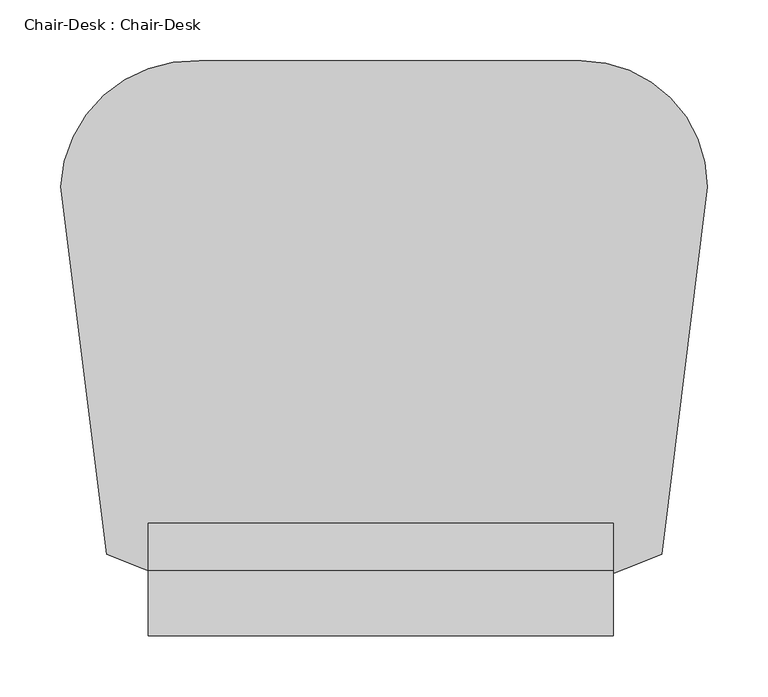
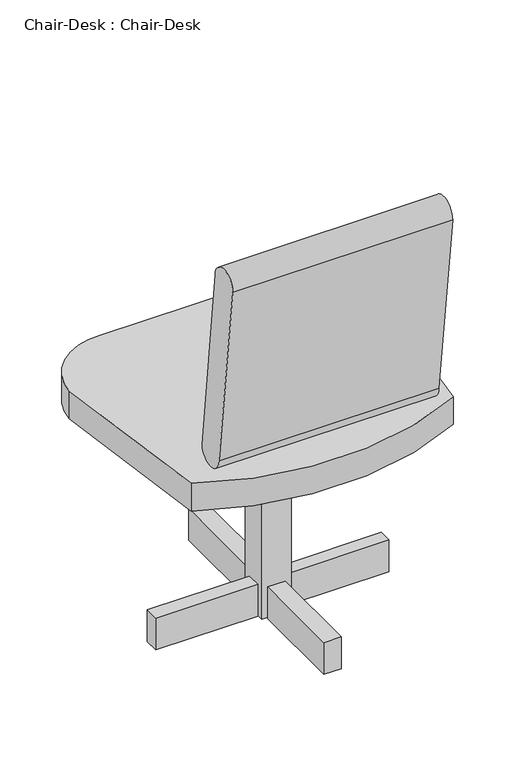
"""IFC4 building model written with IfcOpenShell, lengths in millimetres: furniture geometry, Chair-Desk : Chair-Desk."""

from ifc_helpers import new_model, si_unit, point, frame, frame_2d, origin, origin_with_axes, place, context, project, spatial, polyline, circle_curve, trimmed, segment, composite_curve, outline, extrude, source, transform, mapped, element, save


def chair_desk_chair_desk_7ad88740(model_context):
    return source(origin(), model_context, "Body", "SweptSolid", [
        extrude(outline(composite_curve([segment(trimmed(circle_curve(frame_2d((-157.1362322, 297.1024212)), 109.4001491), [point((-266.4057871, 302.4462968))], [point((-152.4, 406.4))], False, "CARTESIAN"), True, "CONTINUOUS"), segment(polyline([(-152.4, 406.4), (162.2530084, 406.4)]), True, "CONTINUOUS"), segment(trimmed(circle_curve(frame_2d((162.2530084, 302.4462968)), 103.9537032), [point((162.2530084, 406.4))], [point((266.2067116, 302.4462968))], False, "CARTESIAN"), True, "CONTINUOUS"), segment(polyline([(266.2067116, 302.4462968), (228.6, 0.0)]), True, "CONTINUOUS"), segment(trimmed(circle_curve(frame_2d((0.0, 446.8941036)), 501.9684252), [point((228.6, 0.0))], [point((-228.6, 0.0))], False, "CARTESIAN"), True, "CONTINUOUS"), segment(polyline([(-228.6, 0.0), (-266.4057871, 302.4462968)]), True, "CONTINUOUS")], self_intersect=False)), frame((0.0, 0.0, 355.6), z_axis=(0.0, 0.0, 1.0), x_axis=(1.0, 0.0, 0.0)), (0.0, 0.0, 1.0), 50.8),
        extrude(outline(composite_curve([segment(polyline([(-13.6321252, 787.4), (25.5523927, 451.3880753)]), True, "CONTINUOUS"), segment(trimmed(circle_curve(frame_2d((0.0761963, 451.3880753)), 25.4761963), [point((25.5523927, 451.3880753))], [point((-25.4, 451.3880753))], False, "CARTESIAN"), True, "CONTINUOUS"), segment(polyline([(-25.4, 451.3880753), (-67.209111, 787.4)]), True, "CONTINUOUS"), segment(trimmed(circle_curve(frame_2d((-40.4206181, 787.4)), 26.7884929), [point((-67.209111, 787.4))], [point((-13.6321252, 787.4))], False, "CARTESIAN"), True, "CONTINUOUS")], self_intersect=False)), frame((-194.3643056, 0.0, 0.0), z_axis=(1.0, 0.0, 0.0), x_axis=(0.0, 1.0, 0.0)), (0.0, 0.0, 1.0), 383.2768056),
        extrude(outline(polyline([(26.3236364, 190.2690909), (26.3236364, 139.4690909), (-24.4763636, 139.4690909), (-24.4763636, 190.2690909), (26.3236364, 190.2690909)])), origin_with_axes(), (0.0, 0.0, 1.0), 355.6),
        extrude(outline(polyline([(-203.6618182, 175.0290909), (-25.8618182, 175.0290909), (-25.8618182, 150.0462968), (-203.6618182, 150.0462968), (-203.6618182, 175.0290909)])), origin_with_axes(), (0.0, 0.0, 1.0), 58.5040426),
        extrude(outline(polyline([(204.1236364, 175.0290909), (204.1236364, 152.4), (26.7854545, 152.4), (26.7854545, 175.0290909), (204.1236364, 175.0290909)])), origin_with_axes(), (0.0, 0.0, 1.0), 58.5040426),
        extrude(outline(polyline([(-16.1636364, 188.8836364), (-16.1636364, 374.9517514), (14.3163636, 374.9517514), (14.3163636, 188.8836364), (-16.1636364, 188.8836364)])), origin_with_axes(), (0.0, 0.0, 1.0), 58.5040426),
        extrude(outline(polyline([(14.3163636, 136.2363636), (14.3163636, -33.2509091), (-16.1636364, -33.2509091), (-16.1636364, 136.2363636), (14.3163636, 136.2363636)])), origin_with_axes(), (0.0, 0.0, 1.0), 58.5040426),
    ])


if __name__ == "__main__":
    model = new_model("IFC4")
    model_context = context("Model", 3, world=origin())
    ifc_project = project(units=[si_unit("LENGTHUNIT", "METRE", prefix="MILLI")], contexts=[model_context])
    site = spatial("IfcSite", under=ifc_project)
    building = spatial("IfcBuilding", under=site)
    placement = place(None, origin())
    chair_desk_chair_desk_shape = chair_desk_chair_desk_7ad88740(model_context)
    element("IfcFurniture", 1, ObjectType="Chair-Desk : Chair-Desk", at=placement, inside=building, context=model_context, shape_type="MappedRepresentation", body=[
        mapped(chair_desk_chair_desk_shape, transform((0.0, 0.0, 0.0), x_axis=(1.0, 0.0, 0.0), y_axis=(0.0, 1.0, 0.0), z_axis=(0.0, 0.0, 1.0))),
    ])
    save(model, "model.ifc")

# Revit data of these elements
# Type "Chair-Desk : Chair-Desk"
#   Assembly Code = "E2020200"
#   Seat/Back Material = Textile - Slate Blue
#   Base Material = Steel, Chrome Plated
#   Default Elevation = 0
# Element 1 (IfcFurniture, "Chair-Desk : Chair-Desk")
#   Materials on its faces: "Steel, Chrome Plated", "Textile - Slate Blue"
# Materials
#   "Textile - Slate Blue": class "Fabric", colour RGB 98 102 118, transparency 0
#   "Steel, Chrome Plated": class "Metal", colour RGB 17 17 17, transparency 0, Description = "Chromiuim plated steel", Cost = 0
